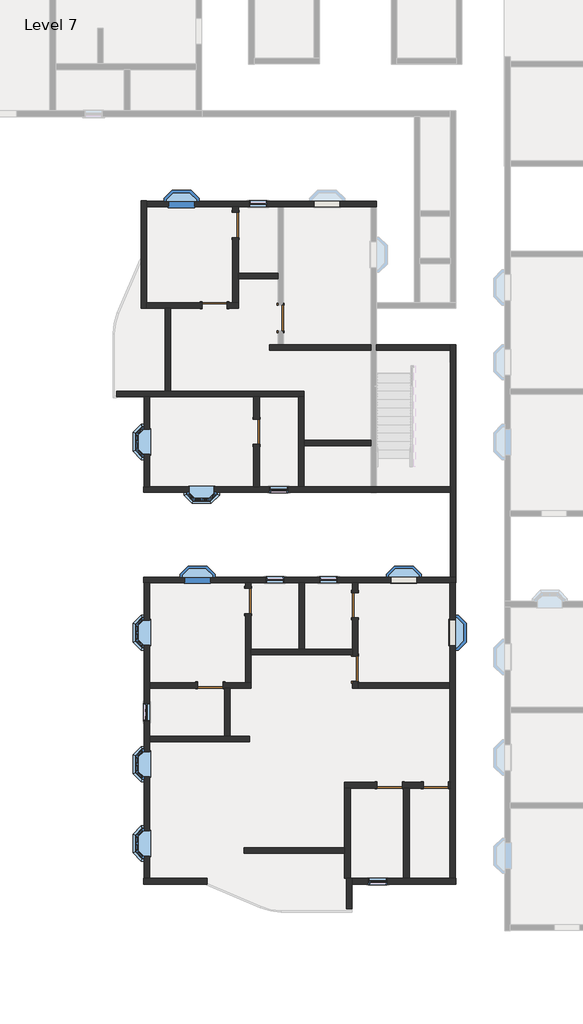
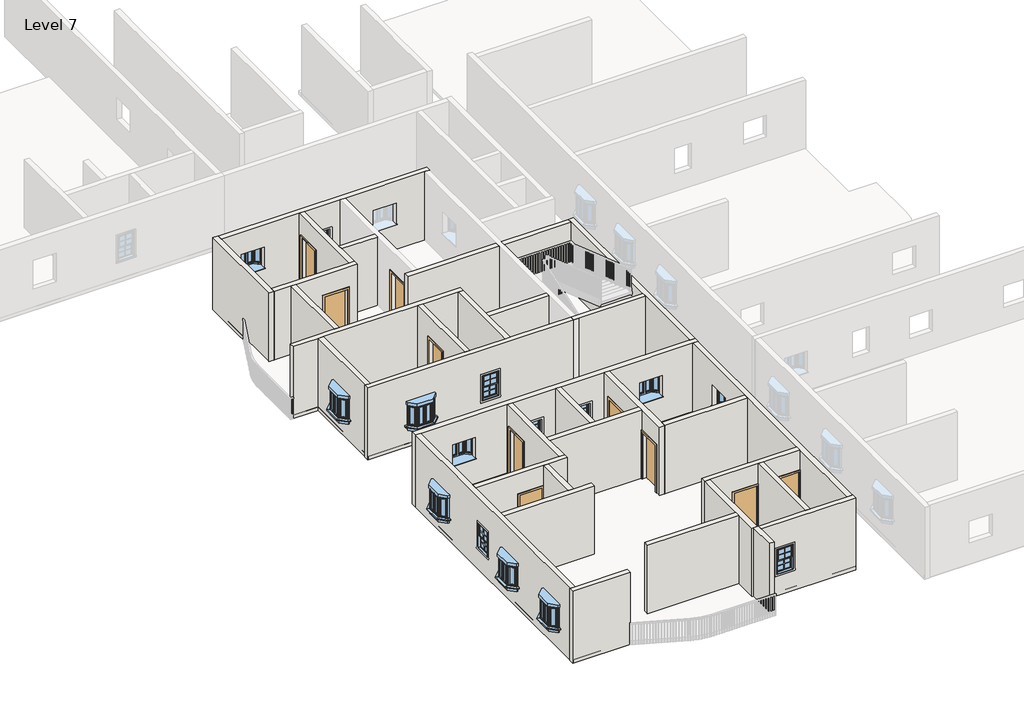
# One storey, part 1 of 14: 32 walls, 15 windows, 10 doors.
# Revit data of these elements (continued)
# Element 54 (IfcWindow, "Window-Double-Hung : 26\" x 42\"") (continued)
#   Window Inset = 0' - 0"
#   Interior Wall Closure = 0' - 1 1/2"
#   Frame Extension = 0' - 1 1/4"
#   Exterior Wall Closure = 0' - 0 1/2"
#   Interior Trim Visibility = yes
#   Indicator Visibility = yes
#   Exterior Trim Visibility = yes
#   Phase Created = New Construction
#   Materials on its faces: "Wood - Stained", "Glass", "Clad - White"
# Element 55 (IfcWindow, "Window-Double-Hung : 26\" x 42\"")
#   Mark = "408"
#   Window Inset = 0' - 0"
#   Interior Wall Closure = 0' - 1 1/2"
#   Frame Extension = 0' - 1 1/4"
#   Exterior Wall Closure = 0' - 0 1/2"
#   Interior Trim Visibility = yes
#   Indicator Visibility = yes
#   Exterior Trim Visibility = yes
#   Phase Created = New Construction
#   Materials on its faces: "Wood - Stained", "Glass", "Clad - White"
# Element 56 (IfcWindow, "Window-Double-Hung : 26\" x 42\"")
#   Mark = "409"
#   Window Inset = 0' - 0"
#   Interior Wall Closure = 0' - 1 1/2"
#   Frame Extension = 0' - 1 1/4"
#   Exterior Wall Closure = 0' - 0 1/2"
#   Interior Trim Visibility = yes
#   Indicator Visibility = yes
#   Exterior Trim Visibility = yes
#   Phase Created = New Construction
#   Materials on its faces: "Wood - Stained", "Glass", "Clad - White"
# Element 57 (IfcWindow, "Window-Double-Hung : 26\" x 42\"")
#   Mark = "410"
#   Window Inset = 0' - 0"
#   Interior Wall Closure = 0' - 1 1/2"
#   Frame Extension = 0' - 1 1/4"
#   Exterior Wall Closure = 0' - 0 1/2"
#   Interior Trim Visibility = yes
#   Indicator Visibility = yes
#   Exterior Trim Visibility = yes
#   Phase Created = New Construction
#   Materials on its faces: "Wood - Stained", "Glass", "Clad - White"
# Materials
#   "Door - Panel": class "Wood", colour RGB 210 159 95, transparency 0, Cost = 0
#   "Door - Frame": colour RGB 118 70 51, transparency 0, Cost = 0
#   "Window Frame": colour RGB 249 249 249, transparency 0
#   "Glass": class "Glass", colour RGB 0 128 192, transparency 0.75, Description = "Soda Lime Glass", Cost = 0
#   "Wood - Stained": class "Wood", colour RGB 224 178 126, transparency 0, Cost = 0
#   "Clad - White": class "Wood", colour RGB 242 242 238, transparency 0, Cost = 0
#   "Default Wall": colour RGB 128 128 128, transparency 0, Cost = 0
#   "Earth": class "Generic", colour RGB 97 75 62, transparency 0, Description = "Soil", Cost = 0
#   "Parking Stripe": class "Paint", colour RGB 250 250 91, transparency 0, Cost = 0
#   "Carpet (1)": class "Carpet", colour RGB 124 80 67, transparency 0, Description = "Interior finish", Cost = 0
#   "Softwood, Lumber": class "Wood", colour RGB 223 192 134, transparency 0, Description = "Pinus Echinata", Cost = 0
